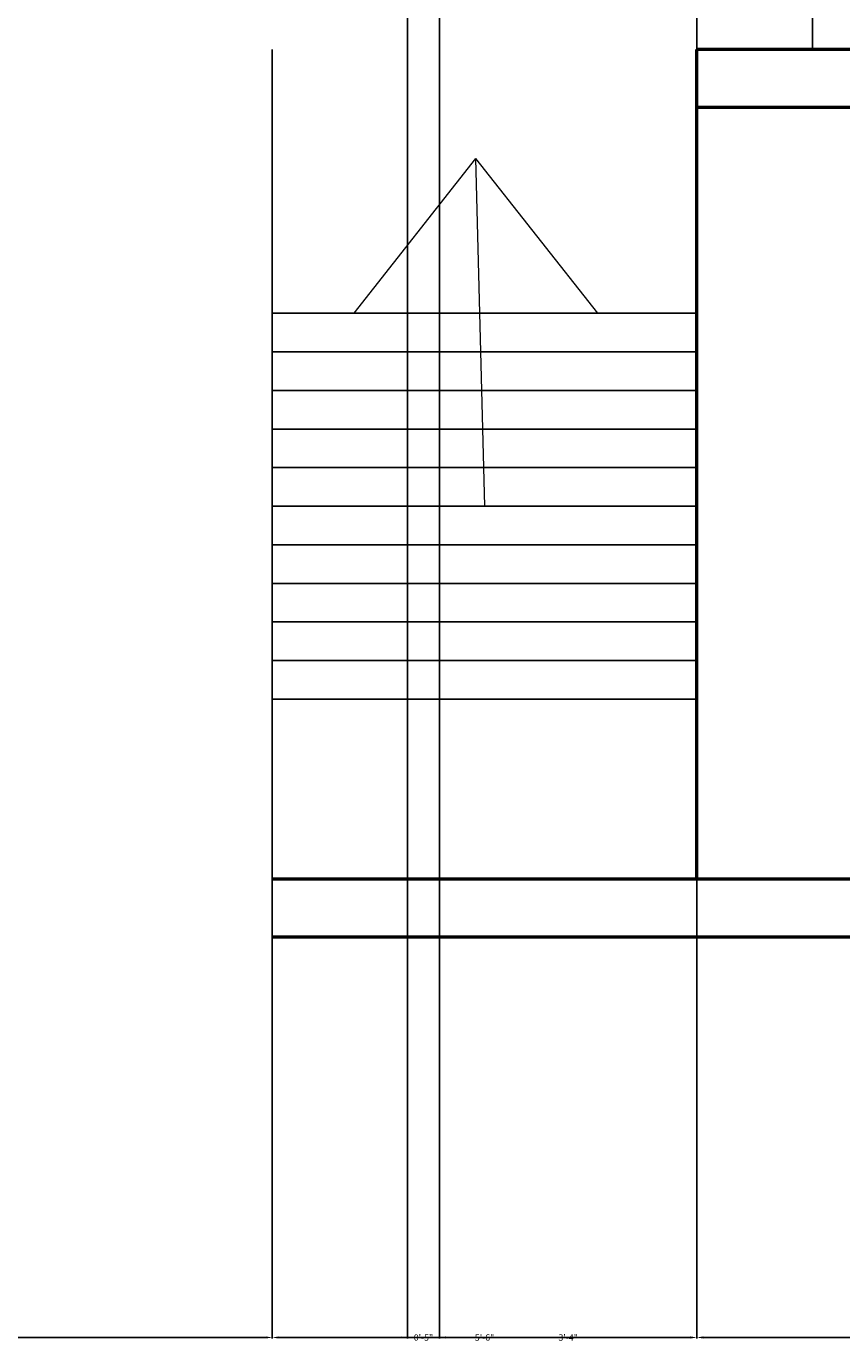
# Model space of a CAD drawing. Units: inches. Extents: x -364 to 705, y -52 to 1250.
# Tile 11 of 34: x 308 to 435, y -52 to 153. Entities that reach past the tile are written whole.
import ezdxf

# ---------------------------------------------------------------- set-up
doc = ezdxf.new("R2010")
doc.units = ezdxf.units.IN
doc.header["$MEASUREMENT"] = 0
for name, color, linetype, lineweight in [('A-ANNO-DIMS', 4, 'Continuous', 18), ('A-ANNO-SYMB', 7, 'Continuous', 18), ('A-FLOR-RAMP', 7, 'Continuous', 25), ('A-FLOR-STRS', 7, 'Continuous', 25), ('A-WALL', 41, 'Continuous', 50)]:
    doc.layers.add(name, color=color, linetype=linetype, lineweight=lineweight)
doc.styles.get("Standard").update_dxf_attribs({"font": 'arial.ttf'})
doc.dimstyles.get("Standard").update_dxf_attribs({"dimtxt": 1, "dimasz": 1, "dimexe": 0.18, "dimexo": 0.0625, "dimgap": 0.09, "dimtad": 0, "dimtih": 1, "dimtoh": 1, "dimdec": 0, "dimzin": 0, "dimdsep": 46, "dimlunit": 3, "dimtxsty": 'Standard', "dimcen": 0.09, "dimadec": 0, "dimazin": 0, "dimtfac": 1, "dimtdec": 0, "dimtofl": 0, "dimtmove": 0, "dimatfit": 3, "dimfxl": 1, "dimtolj": 1, "dimtzin": 0, "dimarcsym": 0})

# ---------------------------------------------------------------- blocks, each defined once
blk = doc.blocks.new('STAIR-DIRECTION')
for q in [(0, 30), (20.33, 0), (37.87, 30)]:
    blk.add_line((18.93, 54.04), q)
blk = doc.blocks.new('*D87')
at = {"layer": 'A-ANNO-DIMS', "color": 0, "lineweight": -2, "transparency": 16777216}
for p, q in [((226.58, 11.05), (226.58, -51.32)), ((346.58, 11.05), (346.58, -51.32)), ((227.58, -51.14), (284.82, -51.14)), ((345.58, -51.14), (288.34, -51.14))]:
    blk.add_line(p, q, dxfattribs=at)
at = {"layer": 'A-ANNO-DIMS', "color": 0, "transparency": 16777216}
for points in [[(227.58, -50.97), (227.58, -51.3), (226.58, -51.14)], [(345.58, -50.97), (345.58, -51.3), (346.58, -51.14)]]:
    blk.add_solid(points, dxfattribs=at)
at = {"layer": 'Defpoints', "color": 0, "transparency": 16777216}
for p in [(226.58, 11.11), (346.58, 11.11), (346.58, -51.14)]:
    blk.add_point(p, dxfattribs=at)
at = {"layer": 'A-ANNO-DIMS', "color": 0, "transparency": 16777216, "insert": (286.58, -51.14), "char_height": 1, "attachment_point": 5}
blk.add_mtext('\\A1;10\'-0"', dxfattribs=at)
blk = doc.blocks.new('*D88')
at = {"layer": 'A-ANNO-DIMS', "color": 0, "lineweight": -2, "transparency": 16777216}
for p, q in [((412.58, 20.05), (412.58, -51.32)), ((346.58, 11.05), (346.58, -51.32)), ((347.58, -51.14), (378.16, -51.14)), ((411.58, -51.14), (381, -51.14))]:
    blk.add_line(p, q, dxfattribs=at)
at = {"layer": 'A-ANNO-DIMS', "color": 0, "transparency": 16777216}
for points in [[(347.58, -50.97), (347.58, -51.3), (346.58, -51.14)], [(411.58, -50.97), (411.58, -51.3), (412.58, -51.14)]]:
    blk.add_solid(points, dxfattribs=at)
at = {"layer": 'Defpoints', "color": 0, "transparency": 16777216}
for p in [(412.58, 20.11), (346.58, 11.11), (412.58, -51.14)]:
    blk.add_point(p, dxfattribs=at)
at = {"layer": 'A-ANNO-DIMS', "color": 0, "transparency": 16777216, "insert": (379.58, -51.14), "char_height": 1, "attachment_point": 5}
blk.add_mtext('\\A1;5\'-6"', dxfattribs=at)
blk = doc.blocks.new('*D89')
at = {"layer": 'A-ANNO-DIMS', "color": 0, "lineweight": -2, "transparency": 16777216}
for p, q in [((412.58, 20.05), (412.58, -51.32)), ((547.58, 11.05), (547.58, -51.32)), ((413.58, -51.14), (478.32, -51.14)), ((546.58, -51.14), (481.84, -51.14))]:
    blk.add_line(p, q, dxfattribs=at)
at = {"layer": 'A-ANNO-DIMS', "color": 0, "transparency": 16777216}
for points in [[(413.58, -50.97), (413.58, -51.3), (412.58, -51.14)], [(546.58, -50.97), (546.58, -51.3), (547.58, -51.14)]]:
    blk.add_solid(points, dxfattribs=at)
at = {"layer": 'Defpoints', "color": 0, "transparency": 16777216}
for p in [(412.58, 20.11), (547.58, 11.11), (547.58, -51.14)]:
    blk.add_point(p, dxfattribs=at)
at = {"layer": 'A-ANNO-DIMS', "color": 0, "transparency": 16777216, "insert": (480.08, -51.14), "char_height": 1, "attachment_point": 5}
blk.add_mtext('\\A1;11\'-3"', dxfattribs=at)
blk = doc.blocks.new('*D101')
at = {"layer": 'A-ANNO-DIMS', "color": 0, "lineweight": -2, "transparency": 16777216}
for p, q in [((372.58, 408.05), (372.58, -51.32)), ((412.58, 408.05), (412.58, -51.32)), ((373.58, -51.14), (391.16, -51.14)), ((411.58, -51.14), (394, -51.14))]:
    blk.add_line(p, q, dxfattribs=at)
at = {"layer": 'A-ANNO-DIMS', "color": 0, "transparency": 16777216}
for points in [[(373.58, -50.97), (373.58, -51.3), (372.58, -51.14)], [(411.58, -50.97), (411.58, -51.3), (412.58, -51.14)]]:
    blk.add_solid(points, dxfattribs=at)
at = {"layer": 'Defpoints', "color": 0, "transparency": 16777216}
for p in [(372.58, 408.11), (412.58, 408.11), (412.58, -51.14)]:
    blk.add_point(p, dxfattribs=at)
at = {"layer": 'A-ANNO-DIMS', "color": 0, "transparency": 16777216, "insert": (392.58, -51.14), "char_height": 1, "attachment_point": 5}
blk.add_mtext('\\A1;3\'-4"', dxfattribs=at)
blk = doc.blocks.new('*D102')
at = {"layer": 'A-ANNO-DIMS', "color": 0, "lineweight": -2, "transparency": 16777216}
for p, q in [((367.58, 408.05), (367.58, -51.32)), ((372.58, 408.05), (372.58, -51.32)), ((366.58, -51.14), (365.58, -51.14)), ((373.58, -51.14), (374.58, -51.14))]:
    blk.add_line(p, q, dxfattribs=at)
at = {"layer": 'A-ANNO-DIMS', "color": 0, "transparency": 16777216}
for points in [[(366.58, -50.97), (366.58, -51.3), (367.58, -51.14)], [(373.58, -50.97), (373.58, -51.3), (372.58, -51.14)]]:
    blk.add_solid(points, dxfattribs=at)
at = {"layer": 'Defpoints', "color": 0, "transparency": 16777216}
for p in [(367.58, 408.11), (372.58, 408.11), (372.58, -51.14)]:
    blk.add_point(p, dxfattribs=at)
at = {"layer": 'A-ANNO-DIMS', "color": 0, "transparency": 16777216, "insert": (370.08, -51.14), "char_height": 1, "attachment_point": 5}
blk.add_mtext('\\A1;0\'-5"', dxfattribs=at)

msp = doc.modelspace()

# ---------------------------------------------------------------- linework, layer by layer
at = {"layer": 'A-FLOR-RAMP'}
msp.add_line((346.58, 11.11), (346.58, 149.11), dxfattribs=at)
at = {"layer": 'A-FLOR-STRS'}
for p, q in [((430.58, 190.11), (430.58, 149.11)), ((412.58, 108.1), (346.58, 108.1)), ((412.58, 102.1), (346.58, 102.1)), ((412.58, 96.1), (346.58, 96.1)), ((412.58, 90.1), (346.58, 90.1)), ((412.58, 84.1), (346.58, 84.1)), ((412.58, 78.1), (346.58, 78.1)), ((412.58, 72.1), (346.58, 72.1)), ((412.58, 66.1), (346.58, 66.1)), ((412.58, 60.1), (346.58, 60.1)), ((412.58, 54.1), (346.58, 54.1)), ((412.58, 48.1), (346.58, 48.1))]:
    msp.add_line(p, q, dxfattribs=at)
at = {"layer": 'A-WALL'}
for p, q in [((547.58, 149.11), (412.58, 149.11)), ((412.58, 20.11), (412.58, 149.11)), ((547.58, 140.11), (412.58, 140.11)), ((538.58, 20.11), (346.58, 20.11)), ((547.58, 11.11), (346.58, 11.11))]:
    msp.add_line(p, q, dxfattribs=at)

# ---------------------------------------------------------------- block references
at = {"layer": 'A-ANNO-SYMB'}
msp.add_blockref('STAIR-DIRECTION', (359.25, 78.1), dxfattribs=at)

# ---------------------------------------------------------------- dimensions: what is measured, and where the dimension line sits
at = {"layer": 'A-ANNO-DIMS'}
for base, p1, p2, picture, middle in [((372.58, -51.14), (367.58, 408.11), (372.58, 408.11), '*D102', (370.08, -51.14)), ((412.58, -51.14), (372.58, 408.11), (412.58, 408.11), '*D101', (392.58, -51.14)), ((412.58, -51.14), (346.58, 11.11), (412.58, 20.11), '*D88', (379.58, -51.14)), ((547.58, -51.14), (412.58, 20.11), (547.58, 11.11), '*D89', (480.08, -51.14)), ((346.58, -51.14), (226.58, 11.11), (346.58, 11.11), '*D87', (286.58, -51.14))]:
    dim = msp.add_linear_dim(base=base, p1=p1, p2=p2, dimstyle='Standard', override={"dimdec": 1, "dimlfac": 1, "dimrnd": 0, "dimzin": 1, "dimdsep": 46, "dimlunit": 4, "dimfrac": 2}, dxfattribs=at)
    dim.commit()
    dim.dimension.update_dxf_attribs({"geometry": picture, "text_midpoint": middle})

doc.saveas('drawing.dxf')
